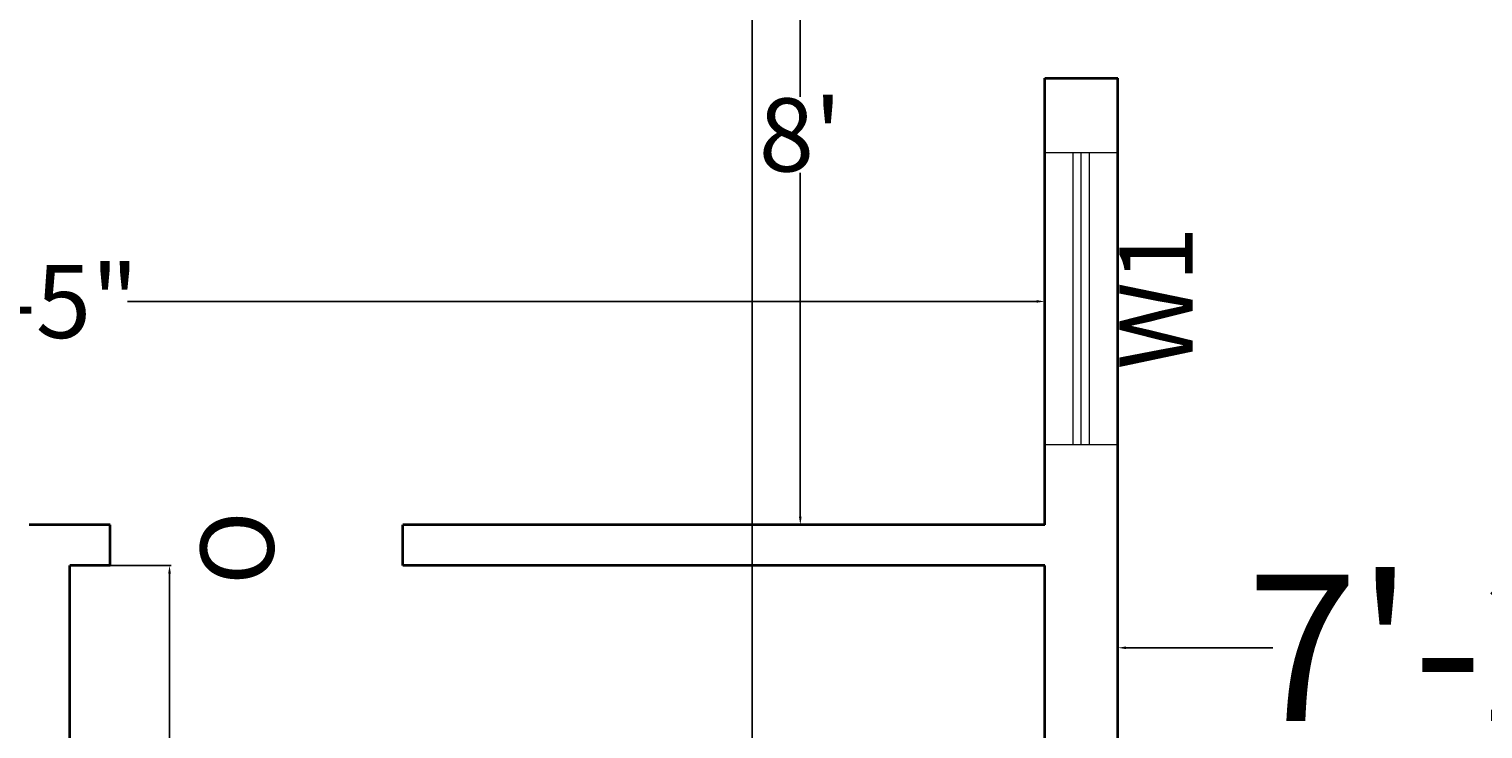
# Model space of a CAD drawing. Units: inches. Extents: x -2189 to 546, y 945 to 2684.
# Tile 7 of 10: x -492 to -313, y 2366 to 2452. Entities that reach past the tile are written whole.
import ezdxf

# ---------------------------------------------------------------- set-up
doc = ezdxf.new("R2010")
doc.units = ezdxf.units.IN
doc.header["$MEASUREMENT"] = 0
for name, color, linetype, lineweight in [('A-ANNO-DIMS', 2, 'Continuous', 13), ('A-ANNO-TEXT', 7, 'Continuous', 18), ('A-GLAZ', 4, 'Continuous', 18), ('A-WALL', 7, 'Continuous', 35)]:
    doc.layers.add(name, color=color, linetype=linetype, lineweight=lineweight)
doc.styles.get("Standard").update_dxf_attribs({"font": 'arial.ttf'})
doc.dimstyles.get("Standard").update_dxf_attribs({"dimtxt": 1, "dimasz": 1, "dimexe": 0.18, "dimexo": 0.0625, "dimgap": 0.09, "dimtad": 0, "dimtih": 1, "dimtoh": 1, "dimdec": 0, "dimzin": 0, "dimdsep": 46, "dimlunit": 3, "dimtxsty": 'Standard', "dimcen": 0.09, "dimadec": 0, "dimazin": 0, "dimtfac": 1, "dimtdec": 0, "dimtofl": 0, "dimtmove": 0, "dimatfit": 3, "dimfxl": 1, "dimtolj": 1, "dimtzin": 0, "dimarcsym": 0})

# ---------------------------------------------------------------- blocks, each defined once
blk = doc.blocks.new('*D70')
at = {"layer": 'A-ANNO-DIMS', "color": 0, "lineweight": -2, "transparency": 16777216}
for p, q in [((-486.72, 2386.17), (-474.31, 2386.17)), ((-474.49, 2385.17), (-474.49, 2342.86)), ((-474.49, 2291.17), (-474.49, 2333.49)), ((-486.72, 2290.17), (-474.31, 2290.17))]:
    blk.add_line(p, q, dxfattribs=at)
at = {"layer": 'A-ANNO-DIMS', "color": 0, "transparency": 16777216}
for points in [[(-474.66, 2385.17), (-474.33, 2385.17), (-474.49, 2386.17)], [(-474.66, 2291.17), (-474.33, 2291.17), (-474.49, 2290.17)]]:
    blk.add_solid(points, dxfattribs=at)
at = {"layer": 'Defpoints', "color": 0, "transparency": 16777216}
for p in [(-486.78, 2386.17), (-486.78, 2290.17), (-474.49, 2290.17)]:
    blk.add_point(p, dxfattribs=at)
at = {"layer": 'A-ANNO-DIMS', "color": 0, "transparency": 16777216, "insert": (-474.49, 2338.17), "char_height": 1, "attachment_point": 5}
blk.add_mtext("\\A1;{\\H9x;8'}", dxfattribs=at)
blk = doc.blocks.new('*D77')
at = {"layer": 'A-ANNO-DIMS', "color": 0, "lineweight": -2, "transparency": 16777216}
for p, q in [((-623.78, 2415.24), (-623.78, 2418.85)), ((-622.78, 2418.67), (-510.9, 2418.67)), ((-367.78, 2418.67), (-479.65, 2418.67)), ((-366.78, 2415.24), (-366.78, 2418.85))]:
    blk.add_line(p, q, dxfattribs=at)
at = {"layer": 'A-ANNO-DIMS', "color": 0, "transparency": 16777216}
for points in [[(-622.78, 2418.84), (-622.78, 2418.51), (-623.78, 2418.67)], [(-367.78, 2418.84), (-367.78, 2418.51), (-366.78, 2418.67)]]:
    blk.add_solid(points, dxfattribs=at)
at = {"layer": 'Defpoints', "color": 0, "transparency": 16777216}
for p in [(-366.78, 2418.67), (-623.78, 2415.17), (-366.78, 2415.17)]:
    blk.add_point(p, dxfattribs=at)
at = {"layer": 'A-ANNO-DIMS', "color": 0, "transparency": 16777216, "insert": (-495.28, 2418.67), "char_height": 1, "attachment_point": 5}
blk.add_mtext('\\A1;{\\H9x;21\'-5"}', dxfattribs=at)
blk = doc.blocks.new('*D78')
at = {"layer": 'A-ANNO-DIMS', "color": 0, "lineweight": -2, "transparency": 16777216}
for p, q in [((-366.84, 2487.17), (-397.04, 2487.17)), ((-396.86, 2486.17), (-396.86, 2443.86)), ((-396.86, 2392.17), (-396.86, 2434.49)), ((-366.84, 2391.17), (-397.04, 2391.17))]:
    blk.add_line(p, q, dxfattribs=at)
at = {"layer": 'A-ANNO-DIMS', "color": 0, "transparency": 16777216}
for points in [[(-397.03, 2486.17), (-396.7, 2486.17), (-396.86, 2487.17)], [(-397.03, 2392.17), (-396.7, 2392.17), (-396.86, 2391.17)]]:
    blk.add_solid(points, dxfattribs=at)
at = {"layer": 'Defpoints', "color": 0, "transparency": 16777216}
for p in [(-396.86, 2487.17), (-366.78, 2487.17), (-366.78, 2391.17)]:
    blk.add_point(p, dxfattribs=at)
at = {"layer": 'A-ANNO-DIMS', "color": 0, "transparency": 16777216, "insert": (-396.86, 2439.17), "char_height": 1, "attachment_point": 5}
blk.add_mtext("\\A1;{\\H9x;8'}", dxfattribs=at)
blk = doc.blocks.new('*D83')
at = {"layer": 'A-ANNO-DIMS', "color": 0, "lineweight": -2, "transparency": 16777216}
for p, q in [((-357.78, 2376.1), (-357.78, 2376.22)), ((-271.78, 2376.1), (-271.78, 2376.22)), ((-356.78, 2376.04), (-338.72, 2376.04)), ((-272.78, 2376.04), (-290.84, 2376.04))]:
    blk.add_line(p, q, dxfattribs=at)
at = {"layer": 'A-ANNO-DIMS', "color": 0, "transparency": 16777216}
for points in [[(-356.78, 2376.2), (-356.78, 2375.87), (-357.78, 2376.04)], [(-272.78, 2376.2), (-272.78, 2375.87), (-271.78, 2376.04)]]:
    blk.add_solid(points, dxfattribs=at)
at = {"layer": 'Defpoints', "color": 0, "transparency": 16777216}
for p in [(-357.78, 2376.04), (-271.78, 2376.04), (-271.78, 2376.04)]:
    blk.add_point(p, dxfattribs=at)
at = {"layer": 'A-ANNO-DIMS', "color": 0, "transparency": 16777216, "insert": (-314.78, 2376.04), "char_height": 1, "attachment_point": 5}
blk.add_mtext('\\A1;{\\H18x;7\'-2"}', dxfattribs=at)
blk = doc.blocks.new('WIN-36X9')
for p, q in [((0, 5.5), (36, 5.5)), ((0, 5.5), (36, 5.5)), ((0, 4.5), (36, 4.5)), ((0, 3.5), (36, 3.5))]:
    blk.add_line(p, q)
blk.add_lwpolyline([(0, 0), (0, 9), (36, 9), (36, 0)], close=True)
blk = doc.blocks.new('*D104')
at = {"layer": 'A-ANNO-DIMS', "color": 0, "lineweight": -2, "transparency": 16777216}
for p, q in [((-493.78, 1873.24), (-493.78, 2683.65)), ((-492.78, 2683.47), (-449.69, 2683.47)), ((-403.78, 2683.47), (-446.86, 2683.47)), ((-402.78, 1873.24), (-402.78, 2683.65))]:
    blk.add_line(p, q, dxfattribs=at)
at = {"layer": 'A-ANNO-DIMS', "color": 0, "transparency": 16777216}
for points in [[(-492.78, 2683.64), (-492.78, 2683.31), (-493.78, 2683.47)], [(-403.78, 2683.64), (-403.78, 2683.31), (-402.78, 2683.47)]]:
    blk.add_solid(points, dxfattribs=at)
at = {"layer": 'Defpoints', "color": 0, "transparency": 16777216}
for p in [(-402.78, 2683.47), (-493.78, 1873.17), (-402.78, 1873.17)]:
    blk.add_point(p, dxfattribs=at)
at = {"layer": 'A-ANNO-DIMS', "color": 0, "transparency": 16777216, "insert": (-448.28, 2683.47), "char_height": 1, "attachment_point": 5}
blk.add_mtext('\\A1;7\'-7"', dxfattribs=at)

msp = doc.modelspace()

# ---------------------------------------------------------------- linework, layer by layer
at = {"layer": 'A-WALL'}
for p, q in [((-366.78, 2391.17), (-366.78, 2446.17)), ((-366.78, 2446.17), (-357.78, 2446.17)), ((-357.78, 2276.2), (-357.78, 2446.17)), ((-481.78, 2391.17), (-491.78, 2391.17)), ((-481.78, 2386.17), (-481.78, 2391.17)), ((-366.78, 2391.17), (-445.78, 2391.17)), ((-445.78, 2386.17), (-445.78, 2391.17)), ((-486.78, 2290.17), (-486.78, 2386.17)), ((-481.78, 2386.17), (-486.78, 2386.17)), ((-366.78, 2386.17), (-445.78, 2386.17)), ((-366.78, 2290.17), (-366.78, 2386.17))]:
    msp.add_line(p, q, dxfattribs=at)

# ---------------------------------------------------------------- block references
at = {"layer": 'A-GLAZ', "rotation": 90.00000000000142}
msp.add_blockref('WIN-36X9', (-357.78, 2401.01), dxfattribs=at)

# ---------------------------------------------------------------- texts
at = {"layer": 'A-ANNO-TEXT', "char_height": 9, "attachment_point": 1, "rotation": 90}
for s, width, heights, insert in [('W1', 11.3125, [0], (-357.59, 2410.28)), ('O', 18.6541, [0.207], (-470.67, 2383.76))]:
    msp.add_mtext_dynamic_manual_height_columns(s, width=width, gutter_width=1, heights=heights, dxfattribs=dict(at, insert=insert))

# ---------------------------------------------------------------- dimensions: what is measured, and where the dimension line sits
at = {"layer": 'A-ANNO-DIMS'}
dim = msp.add_linear_dim(base=(-402.78, 2683.47), p1=(-493.78, 1873.17), p2=(-402.78, 1873.17), dimstyle='Standard', override={"dimdec": 1, "dimlfac": 1, "dimrnd": 0, "dimzin": 1, "dimdsep": 46, "dimlunit": 4, "dimfrac": 2}, dxfattribs=at)
dim.commit()
dim.dimension.update_dxf_attribs({"geometry": '*D104', "text_midpoint": (-448.28, 2683.47)})
for base, p1, p2, angle, picture, middle in [((-396.86, 2487.17), (-366.78, 2391.17), (-366.78, 2487.17), 90, '*D78', (-396.86, 2439.17)), ((-366.78, 2418.67), (-623.78, 2415.17), (-366.78, 2415.17), 180, '*D77', (-495.28, 2418.67)), ((-474.49, 2290.17), (-486.78, 2386.17), (-486.78, 2290.17), 90, '*D70', (-474.49, 2338.17))]:
    dim = msp.add_linear_dim(base=base, p1=p1, p2=p2, angle=angle, text='{\\H9x;<>}', dimstyle='Standard', override={"dimclrd": 0, "dimclre": 0, "dimclrt": 0}, dxfattribs=at)
    dim.commit()
    dim.dimension.update_dxf_attribs({"geometry": picture, "text_midpoint": middle})
dim = msp.add_linear_dim(base=(-271.78, 2376.04), p1=(-357.78, 2376.04), p2=(-271.78, 2376.04), text='{\\H18x;<>}', dimstyle='Standard', override={"dimclrd": 0, "dimclre": 0, "dimclrt": 0}, dxfattribs=at)
dim.commit()
dim.dimension.update_dxf_attribs({"geometry": '*D83', "text_midpoint": (-314.78, 2376.04)})

doc.saveas('drawing.dxf')
